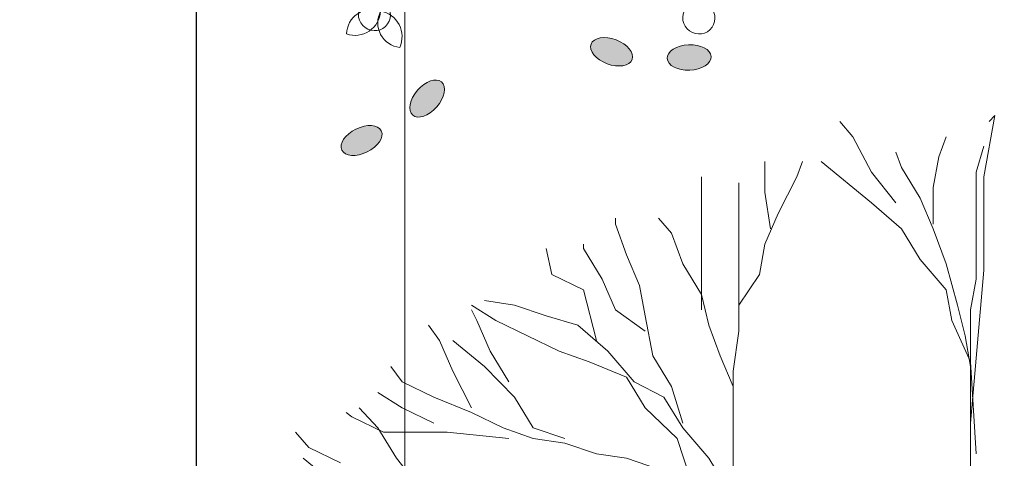
# Model space of a CAD drawing. Units: millimetres. Extents: x 595116 to 630915, y 909473 to 920225.
# Tile 44 of 134: x 629500 to 629529, y 919242 to 919255. Entities that reach past the tile are written whole.
import ezdxf

# ---------------------------------------------------------------- set-up
doc = ezdxf.new("R2010")
doc.units = ezdxf.units.MM
doc.layers.add('Dimension', color=3, linetype='Continuous', lineweight=18)
doc.layers.add('L-PLNT', color=85, linetype='Continuous', lineweight=13)
doc.styles.get("Standard").update_dxf_attribs({"font": 'arial.ttf'})
doc.dimstyles.new('ISO-25', dxfattribs={"dimtxt": 9, "dimasz": 6, "dimexe": 1.25, "dimexo": 0.625, "dimtad": 1, "dimlunit": 4, "dimtxsty": 'Standard', "dimcen": 2.5, "dimadec": 0, "dimazin": 0, "dimtfac": 1, "dimtmove": 0, "dimatfit": 3, "dimfxl": 1, "dimarcsym": 0})

# ---------------------------------------------------------------- blocks, each defined once
blk = doc.blocks.new('A$C143125F4')
for p, q in [((2.5383, 4.8203), (2.5711, 4.9995)), ((2.5711, 4.9995), (2.5547, 4.9816)), ((2.1554, 4.9368), (2.1171, 4.9816)), ((2.2101, 4.8338), (2.1554, 4.9368)), ((2.407, 4.8786), (2.4289, 4.9368)), ((2.5164, 4.8338), (2.5383, 4.9099)), ((2.2976, 4.8472), (2.2812, 4.892)), ((2.3906, 4.789), (2.407, 4.8786)), ((1.8983, 4.7755), (1.8983, 4.8651)), ((1.9913, 4.8203), (2.0077, 4.8651)), ((2.2101, 4.7442), (2.0624, 4.8651)), ((2.3523, 4.7576), (2.2976, 4.8472)), ((1.7123, 4.4306), (1.7123, 4.8203)), ((1.9366, 4.7128), (1.9913, 4.8203)), ((2.2812, 4.7442), (2.2101, 4.8338)), ((2.5164, 4.5202), (2.5164, 4.8338)), ((2.5383, 4.5471), (2.5383, 4.8203)), ((1.8217, 4.3679), (1.8217, 4.8024)), ((2.3906, 4.6814), (2.3906, 4.789)), ((1.9147, 4.668), (1.8983, 4.7755)), ((2.3906, 4.668), (2.3523, 4.7576)), ((2.2976, 4.668), (2.2101, 4.7442)), ((1.4606, 4.6814), (1.4606, 4.6994)), ((1.6247, 4.6546), (1.5865, 4.6994)), ((1.8983, 4.6232), (1.9366, 4.7128)), ((1.4935, 4.5919), (1.4606, 4.6814)), ((2.3523, 4.5784), (2.2976, 4.668)), ((2.4289, 4.565), (2.3906, 4.668)), ((1.6576, 4.565), (1.6247, 4.6546)), ((1.2746, 4.5336), (1.2582, 4.6098)), ((1.3676, 4.6098), (1.3676, 4.6232)), ((1.4223, 4.5202), (1.3676, 4.6098)), ((1.8819, 4.5336), (1.8983, 4.6232)), ((1.5317, 4.5023), (1.4935, 4.5919)), ((1.7123, 4.4754), (1.6576, 4.565)), ((2.4289, 4.4888), (2.3523, 4.5784)), ((2.4617, 4.444), (2.4289, 4.565)), ((1.3676, 4.4888), (1.2746, 4.5336)), ((1.8217, 4.444), (1.8819, 4.5336)), ((2.5, 4.0991), (2.5383, 4.5471)), ((1.4606, 4.4306), (1.4223, 4.5202)), ((1.5482, 4.4127), (1.5317, 4.5023)), ((2.5, 4.4306), (2.5164, 4.5202)), ((1.4059, 4.341), (1.3676, 4.4888)), ((1.7342, 4.3858), (1.7123, 4.4754)), ((2.4453, 4.3992), (2.4289, 4.4888)), ((1.1105, 4.3992), (1.0394, 4.444)), ((1.0777, 4.4575), (1.1652, 4.444)), ((1.1652, 4.444), (1.2582, 4.4127)), ((2.4836, 4.3544), (2.4617, 4.444)), ((1.0558, 4.3992), (1.0394, 4.4306)), ((1.2582, 4.4127), (1.3512, 4.3858)), ((1.5482, 4.3679), (1.4606, 4.4306)), ((1.57, 4.2962), (1.5482, 4.4127)), ((2.5, 3.4584), (2.5, 4.4306)), ((0.9464, 4.341), (0.9136, 4.3858)), ((1.0941, 4.3096), (1.0558, 4.3992)), ((1.2965, 4.3096), (1.1105, 4.3992)), ((1.3512, 4.3858), (1.4387, 4.3096)), ((1.767, 4.2962), (1.7342, 4.3858)), ((2.5, 4.2783), (2.4453, 4.3992)), ((1.8053, 4.2514), (1.8217, 4.3679)), ((2.5, 4.2648), (2.4836, 4.3544)), ((0.9847, 4.2514), (0.9464, 4.341)), ((1.0777, 4.2648), (0.9847, 4.341)), ((1.1488, 4.22), (1.0941, 4.3096)), ((1.384, 4.2783), (1.2965, 4.3096)), ((1.4387, 4.3096), (1.5153, 4.22)), ((1.6247, 4.2066), (1.57, 4.2962)), ((1.8053, 4.2066), (1.767, 4.2962)), ((0.837, 4.22), (0.8042, 4.2648)), ((1.1652, 4.1752), (1.0777, 4.2648)), ((1.4935, 4.2335), (1.384, 4.2783)), ((2.5164, 4.0095), (2.5, 4.2783)), ((1.0394, 4.1439), (0.9847, 4.2514)), ((1.8053, 3.9064), (1.8053, 4.2514)), ((0.93, 4.1752), (0.837, 4.22)), ((1.5482, 4.1439), (1.4935, 4.2335)), ((1.5153, 4.22), (1.6029, 4.1752)), ((1.6576, 4.0991), (1.6247, 4.2066)), ((0.837, 4.1439), (0.7659, 4.1887)), ((1.0394, 4.1304), (0.93, 4.1752)), ((1.2199, 4.0856), (1.1652, 4.1752)), ((1.6029, 4.1752), (1.6576, 4.0856)), ((0.6893, 4.117), (0.6729, 4.1304)), ((0.7659, 4.0856), (0.7112, 4.1439)), ((0.93, 4.0991), (0.837, 4.1439)), ((1.1324, 4.0856), (1.0394, 4.1304)), ((1.6412, 4.0543), (1.5482, 4.1439)), ((0.7823, 4.0722), (0.6893, 4.117)), ((2.5, 3.996), (2.5, 4.0991)), ((0.5635, 4.0274), (0.5252, 4.0722)), ((0.8206, 3.996), (0.7659, 4.0856)), ((0.9683, 4.0722), (0.7823, 4.0722)), ((1.1488, 4.0543), (0.9683, 4.0722)), ((1.2199, 4.0543), (1.1324, 4.0856)), ((1.3129, 4.0543), (1.2199, 4.0856)), ((1.6576, 4.0856), (1.7342, 3.996)), ((1.3129, 4.0408), (1.2199, 4.0543)), ((1.4059, 4.0095), (1.3129, 4.0408)), ((1.6795, 3.9378), (1.6412, 4.0543)), ((0.6565, 3.9826), (0.5635, 4.0274)), ((1.4935, 3.996), (1.4059, 4.0095)), ((0.6018, 3.9512), (0.5471, 3.996)), ((0.8917, 3.9064), (0.8206, 3.996)), ((1.5865, 3.9647), (1.4935, 3.996)), ((1.7342, 3.996), (1.7889, 3.9064))]:
    blk.add_line(p, q)
blk = doc.blocks.new('A$C77972600')
h = blk.add_hatch(color=256)
edge = h.paths.add_edge_path()
edge.add_ellipse((3.2403, 1.6985), major_axis=(-0.1668, -0.0838), ratio=0.578492, start_angle=0, end_angle=360, ccw=False)
edge = h.paths.add_edge_path()
edge.add_ellipse((4.2796, 1.6084), major_axis=(-0.1206, -0.1425), ratio=0.578492, start_angle=0, end_angle=360, ccw=False)
edge = h.paths.add_edge_path()
edge.add_ellipse((4.7739, 0.881), major_axis=(-0.1747, 0.0657), ratio=0.578492, start_angle=0, end_angle=360, ccw=False)
edge = h.paths.add_edge_path()
edge.add_ellipse((5.4333, 0.8328), major_axis=(-0.1865, -0.008), ratio=0.578492, start_angle=0, end_angle=360, ccw=False)
edge = h.paths.add_edge_path()
edge.add_ellipse((4.6573, 4.2045), major_axis=(-0.1865, -0.008), ratio=0.578492, start_angle=0, end_angle=360, ccw=False)
edge = h.paths.add_edge_path()
edge.add_ellipse((4.556, 3.4032), major_axis=(-0.1865, -0.008), ratio=0.578492, start_angle=0, end_angle=360, ccw=False)
edge = h.paths.add_edge_path()
edge.add_ellipse((4.9297, 3.677), major_axis=(-0.1668, -0.0838), ratio=0.578492, start_angle=0, end_angle=360, ccw=False)
edge = h.paths.add_edge_path()
edge.add_ellipse((3.7756, 2.5742), major_axis=(-0.1206, -0.1425), ratio=0.578492, start_angle=0, end_angle=360, ccw=False)
edge = h.paths.add_edge_path()
edge.add_ellipse((3.1788, 2.8466), major_axis=(-0.1206, -0.1425), ratio=0.578492, start_angle=0, end_angle=360, ccw=False)
edge = h.paths.add_edge_path()
edge.add_ellipse((3.8763, 3.0252), major_axis=(-0.1206, -0.1425), ratio=0.578492, start_angle=0, end_angle=360, ccw=False)
edge = h.paths.add_edge_path()
edge.add_ellipse((2.3609, 1.8217), major_axis=(-0.1865, -0.008), ratio=0.578492, start_angle=0, end_angle=360, ccw=False)
edge = h.paths.add_edge_path()
edge.add_ellipse((3.0627, 1.8578), major_axis=(-0.1865, -0.008), ratio=0.578492, start_angle=0, end_angle=360, ccw=False)
edge = h.paths.add_edge_path()
edge.add_ellipse((2.7605, 2.0535), major_axis=(-0.1865, -0.008), ratio=0.578492, start_angle=0, end_angle=360, ccw=False)
edge = h.paths.add_edge_path()
edge.add_ellipse((2.1439, 3.4246), major_axis=(-0.1668, -0.0838), ratio=0.578492, start_angle=0, end_angle=360, ccw=False)
edge = h.paths.add_edge_path()
edge.add_ellipse((4.2959, 2.0225), major_axis=(-0.1747, 0.0657), ratio=0.578492, start_angle=0, end_angle=360, ccw=False)
edge = h.paths.add_edge_path()
edge.add_ellipse((1.9127, 4.2528), major_axis=(-0.1865, -0.008), ratio=0.578492, start_angle=0, end_angle=360, ccw=False)
edge = h.paths.add_edge_path()
edge.add_ellipse((1.5555, 4.1052), major_axis=(-0.1747, 0.0657), ratio=0.578492, start_angle=0, end_angle=360, ccw=False)
edge = h.paths.add_edge_path()
edge.add_ellipse((0.9962, 4.2695), major_axis=(-0.1865, -0.008), ratio=0.578492, start_angle=0, end_angle=360, ccw=False)
edge = h.paths.add_edge_path()
edge.add_ellipse((1.2179, 3.5926), major_axis=(-0.1747, 0.0657), ratio=0.578492, start_angle=0, end_angle=360, ccw=False)
edge = h.paths.add_edge_path()
edge.add_ellipse((1.6764, 3.6493), major_axis=(-0.1747, 0.0657), ratio=0.578492, start_angle=0, end_angle=360, ccw=False)
edge = h.paths.add_edge_path()
edge.add_ellipse((0.8384, 2.8599), major_axis=(-0.1668, -0.0838), ratio=0.578492, start_angle=0, end_angle=360, ccw=False)
edge = h.paths.add_edge_path()
edge.add_ellipse((0.9659, 2.049), major_axis=(-0.1206, -0.1425), ratio=0.578492, start_angle=0, end_angle=360, ccw=False)
edge = h.paths.add_edge_path()
edge.add_ellipse((1.3147, 2.1383), major_axis=(-0.1206, -0.1425), ratio=0.578492, start_angle=0, end_angle=360, ccw=False)
edge = h.paths.add_edge_path()
edge.add_ellipse((5.4586, 2.9929), major_axis=(-0.1865, -0.008), ratio=0.578492, start_angle=0, end_angle=360, ccw=False)
edge = h.paths.add_edge_path()
edge.add_ellipse((3.4224, 5.3915), major_axis=(-0.1865, -0.008), ratio=0.578492, start_angle=0, end_angle=360, ccw=False)
edge = h.paths.add_edge_path()
edge.add_ellipse((3.7245, 5.1958), major_axis=(-0.1865, -0.008), ratio=0.578492, start_angle=0, end_angle=360, ccw=False)
edge = h.paths.add_edge_path()
edge.add_ellipse((4.5588, 5.4431), major_axis=(-0.1668, -0.0838), ratio=0.578492, start_angle=0, end_angle=360, ccw=False)
edge = h.paths.add_edge_path()
edge.add_ellipse((4.4393, 4.7252), major_axis=(-0.1668, -0.0838), ratio=0.578492, start_angle=0, end_angle=360, ccw=False)
edge = h.paths.add_edge_path()
edge.add_ellipse((4.7087, 5.1006), major_axis=(-0.1668, -0.0838), ratio=0.578492, start_angle=0, end_angle=360, ccw=False)
edge = h.paths.add_edge_path()
edge.add_ellipse((3.7138, 4.6852), major_axis=(-0.1668, -0.0838), ratio=0.578492, start_angle=0, end_angle=360, ccw=False)
h = blk.add_hatch(color=256)
edge = h.paths.add_edge_path()
edge.add_ellipse((4.1652, 1.933), major_axis=(0.1866, 0.0058), ratio=0.578492, start_angle=0, end_angle=360)
edge = h.paths.add_edge_path()
edge.add_ellipse((3.2944, 1.3586), major_axis=(0.1739, -0.0678), ratio=0.578492, start_angle=0, end_angle=360)
edge = h.paths.add_edge_path()
edge.add_ellipse((3.2064, 0.4835), major_axis=(0.1223, 0.141), ratio=0.578492, start_angle=0, end_angle=360)
edge = h.paths.add_edge_path()
edge.add_ellipse((2.6497, 0.127), major_axis=(0.1678, 0.0818), ratio=0.578492, start_angle=0, end_angle=360)
edge = h.paths.add_edge_path()
edge.add_ellipse((1.7252, 3.461), major_axis=(0.1678, 0.0818), ratio=0.578492, start_angle=0, end_angle=360)
edge = h.paths.add_edge_path()
edge.add_ellipse((2.1962, 2.8048), major_axis=(0.1678, 0.0818), ratio=0.578492, start_angle=0, end_angle=360)
edge = h.paths.add_edge_path()
edge.add_ellipse((1.7372, 2.8674), major_axis=(0.1866, 0.0058), ratio=0.578492, start_angle=0, end_angle=360)
edge = h.paths.add_edge_path()
edge.add_ellipse((3.2773, 2.4479), major_axis=(0.1739, -0.0678), ratio=0.578492, start_angle=0, end_angle=360)
edge = h.paths.add_edge_path()
edge.add_ellipse((3.6722, 2.9717), major_axis=(0.1739, -0.0678), ratio=0.578492, start_angle=0, end_angle=360)
edge = h.paths.add_edge_path()
edge.add_ellipse((2.9739, 2.7963), major_axis=(0.1739, -0.0678), ratio=0.578492, start_angle=0, end_angle=360)
edge = h.paths.add_edge_path()
edge.add_ellipse((4.8796, 2.4604), major_axis=(0.1678, 0.0818), ratio=0.578492, start_angle=0, end_angle=360)
edge = h.paths.add_edge_path()
edge.add_ellipse((4.2454, 2.1577), major_axis=(0.1678, 0.0818), ratio=0.578492, start_angle=0, end_angle=360)
edge = h.paths.add_edge_path()
edge.add_ellipse((4.4178, 2.4738), major_axis=(0.1678, 0.0818), ratio=0.578492, start_angle=0, end_angle=360)
edge = h.paths.add_edge_path()
edge.add_ellipse((4.3066, 3.973), major_axis=(0.1866, 0.0058), ratio=0.578492, start_angle=0, end_angle=360)
edge = h.paths.add_edge_path()
edge.add_ellipse((3.0828, 1.7149), major_axis=(0.1223, 0.141), ratio=0.578492, start_angle=0, end_angle=360)
edge = h.paths.add_edge_path()
edge.add_ellipse((4.1152, 4.8113), major_axis=(0.1678, 0.0818), ratio=0.578492, start_angle=0, end_angle=360)
edge = h.paths.add_edge_path()
edge.add_ellipse((4.4995, 4.8518), major_axis=(0.1223, 0.141), ratio=0.578492, start_angle=0, end_angle=360)
edge = h.paths.add_edge_path()
edge.add_ellipse((4.913, 5.2627), major_axis=(0.1678, 0.0818), ratio=0.578492, start_angle=0, end_angle=360)
edge = h.paths.add_edge_path()
edge.add_ellipse((5.0407, 4.562), major_axis=(0.1223, 0.141), ratio=0.578492, start_angle=0, end_angle=360)
edge = h.paths.add_edge_path()
edge.add_ellipse((4.6105, 4.3933), major_axis=(0.1223, 0.141), ratio=0.578492, start_angle=0, end_angle=360)
edge = h.paths.add_edge_path()
edge.add_ellipse((5.7235, 4.0986), major_axis=(0.1866, 0.0058), ratio=0.578492, start_angle=0, end_angle=360)
edge = h.paths.add_edge_path()
edge.add_ellipse((5.9977, 3.3249), major_axis=(0.1739, -0.0678), ratio=0.578492, start_angle=0, end_angle=360)
edge = h.paths.add_edge_path()
edge.add_ellipse((5.6486, 3.2372), major_axis=(0.1739, -0.0678), ratio=0.578492, start_angle=0, end_angle=360)
edge = h.paths.add_edge_path()
edge.add_ellipse((1.5981, 2.014), major_axis=(0.1678, 0.0818), ratio=0.578492, start_angle=0, end_angle=360)
edge = h.paths.add_edge_path()
edge.add_ellipse((2.2453, 5.0931), major_axis=(0.1678, 0.0818), ratio=0.578492, start_angle=0, end_angle=360)
edge = h.paths.add_edge_path()
edge.add_ellipse((2.073, 4.777), major_axis=(0.1678, 0.0818), ratio=0.578492, start_angle=0, end_angle=360)
edge = h.paths.add_edge_path()
edge.add_ellipse((1.2216, 4.5968), major_axis=(0.1866, 0.0058), ratio=0.578492, start_angle=0, end_angle=360)
edge = h.paths.add_edge_path()
edge.add_ellipse((1.6688, 4.0227), major_axis=(0.1866, 0.0058), ratio=0.578492, start_angle=0, end_angle=360)
edge = h.paths.add_edge_path()
edge.add_ellipse((1.253, 4.2244), major_axis=(0.1866, 0.0058), ratio=0.578492, start_angle=0, end_angle=360)
edge = h.paths.add_edge_path()
edge.add_ellipse((2.3257, 4.3332), major_axis=(0.1866, 0.0058), ratio=0.578492, start_angle=0, end_angle=360)
for centre, radius, start, end in [((2.7336, 1.03), 0.2106, 68.14697, 179.32342), ((2.5939, 1.2392), 0.2185, 251.0667, 356.4037), ((2.9982, 1.1271), 0.2106, 152.13841, 263.31486), ((2.7756, 1.0101), 0.2185, 335.05813, 80.39514)]:
    blk.add_arc(centre, radius, start, end)
for centre in [(2.7589, 1.1975), (5.5155, 1.1693)]:
    blk.add_ellipse(centre, major_axis=(-0.0941, 0.1005), ratio=0.985729)
at = {"extrusion": (0, 0, -1)}
blk.add_ellipse((4.7739, 0.881), major_axis=(-0.1747, 0.0657), ratio=0.578492, dxfattribs=at)
blk.add_ellipse((5.4333, 0.8328), major_axis=(-0.1865, -0.008), ratio=0.578492, start_param=3.141593, end_param=9.424778, dxfattribs=at)
for centre, major_axis, start_param, end_param in [((3.2064, 0.4835), (-0.1223, -0.141), 3.141593, 9.424778), ((2.6497, 0.127), (-0.1678, -0.0818), -1.570796, 4.712389)]:
    blk.add_ellipse(centre, major_axis=major_axis, ratio=0.578492, start_param=start_param, end_param=end_param)
blk = doc.blocks.new('*D215')
at = {"layer": 'Defpoints', "color": 0, "transparency": 16777216}
for p in [(629316.041, 919411.828), (629505.041, 919411.828), (629505.041, 918832.378)]:
    blk.add_point(p, dxfattribs=at)
at = {"layer": 'Dimension', "color": 0, "lineweight": -2, "transparency": 16777216}
for p, q in [((629316.041, 919411.203), (629316.041, 918831.128)), ((629505.041, 919411.203), (629505.041, 918831.128)), ((629322.041, 918832.378), (629499.041, 918832.378))]:
    blk.add_line(p, q, dxfattribs=at)
at = {"layer": 'Dimension', "color": 0, "transparency": 16777216}
for points in [[(629322.041, 918833.378), (629322.041, 918831.378), (629316.041, 918832.378)], [(629499.041, 918833.378), (629499.041, 918831.378), (629505.041, 918832.378)]]:
    blk.add_solid(points, dxfattribs=at)
at = {"layer": 'Dimension', "color": 0, "transparency": 16777216, "insert": (629410.541, 918837.598), "char_height": 9, "attachment_point": 5}
blk.add_mtext('15\'-9"', dxfattribs=at)
blk = doc.blocks.new('*D216')
at = {"layer": 'Defpoints', "color": 0, "transparency": 16777216}
for p in [(629505.041, 919411.828), (629743.541, 919411.928), (629743.541, 918832.378)]:
    blk.add_point(p, dxfattribs=at)
at = {"layer": 'Dimension', "color": 0, "lineweight": -2, "transparency": 16777216}
for p, q in [((629505.041, 919411.203), (629505.041, 918831.128)), ((629743.541, 919411.303), (629743.541, 918831.128)), ((629511.041, 918832.378), (629737.541, 918832.378))]:
    blk.add_line(p, q, dxfattribs=at)
at = {"layer": 'Dimension', "color": 0, "transparency": 16777216}
for points in [[(629511.041, 918833.378), (629511.041, 918831.378), (629505.041, 918832.378)], [(629737.541, 918833.378), (629737.541, 918831.378), (629743.541, 918832.378)]]:
    blk.add_solid(points, dxfattribs=at)
at = {"layer": 'Dimension', "color": 0, "transparency": 16777216, "insert": (629624.291, 918837.656), "char_height": 9, "attachment_point": 5}
blk.add_mtext('19\'-10 1/2"', dxfattribs=at)
blk = doc.blocks.new('*D221')
at = {"layer": 'Defpoints', "color": 0, "transparency": 16777216}
for p in [(629511.274, 919302.009), (629155.382, 919160.917), (629511.274, 919160.917)]:
    blk.add_point(p, dxfattribs=at)
at = {"layer": 'Dimension', "color": 0, "lineweight": -2, "transparency": 16777216}
for p, q in [((629510.649, 919302.009), (629154.132, 919302.009)), ((629155.382, 919296.009), (629155.382, 919166.917)), ((629510.649, 919160.917), (629154.132, 919160.917))]:
    blk.add_line(p, q, dxfattribs=at)
at = {"layer": 'Dimension', "color": 0, "transparency": 16777216}
for points in [[(629154.382, 919296.009), (629156.382, 919296.009), (629155.382, 919302.009)], [(629154.382, 919166.917), (629156.382, 919166.917), (629155.382, 919160.917)]]:
    blk.add_solid(points, dxfattribs=at)
at = {"layer": 'Dimension', "color": 0, "transparency": 16777216, "insert": (629150.162, 919231.463), "char_height": 9, "attachment_point": 5, "rotation": 90}
blk.add_mtext('11\'-9"', dxfattribs=at)

msp = doc.modelspace()

# ---------------------------------------------------------------- linework, layer by layer
at = {"layer": 'L-PLNT'}
msp.add_line((629511.274, 919302.009), (629511.274, 919160.917), dxfattribs=at)

# ---------------------------------------------------------------- block references
for name, p, xscale, yscale, zscale in [('A$C77972600', (629500.673, 919251.142), 3.512546757812034, 3.512546757812034, 3.512546757812034), ('A$C143125F4', (629502.654, 919201.332), 10.20167662382051, 10.20167662382051, 10.20167662382051)]:
    msp.add_blockref(name, p, dxfattribs=dict(at, xscale=xscale, yscale=yscale, zscale=zscale))

# ---------------------------------------------------------------- dimensions: what is measured, and where the dimension line sits
at = {"layer": 'Dimension'}
for base, p1, p2, picture, middle in [((629505.041, 918832.378), (629316.041, 919411.828), (629505.041, 919411.828), '*D215', (629410.541, 918837.598)), ((629743.541, 918832.378), (629505.041, 919411.828), (629743.541, 919411.928), '*D216', (629624.291, 918837.656))]:
    dim = msp.add_linear_dim(base=base, p1=p1, p2=p2, dimstyle='ISO-25', override={"dimdec": 1, "dimlfac": 1, "dimrnd": 0, "dimzin": 1, "dimdsep": 46, "dimlunit": 4, "dimfrac": 2}, dxfattribs=at)
    dim.commit()
    dim.dimension.update_dxf_attribs({"geometry": picture, "text_midpoint": middle})
dim = msp.add_linear_dim(base=(629155.382, 919160.917), p1=(629511.274, 919302.009), p2=(629511.274, 919160.917), angle=90, dimstyle='ISO-25', override={"dimdec": 1, "dimlfac": 1, "dimrnd": 0, "dimzin": 1, "dimdsep": 46, "dimlunit": 4, "dimfrac": 2}, dxfattribs=at)
dim.commit()
dim.dimension.update_dxf_attribs({"geometry": '*D221', "text_midpoint": (629150.162, 919231.463)})

doc.saveas('drawing.dxf')
